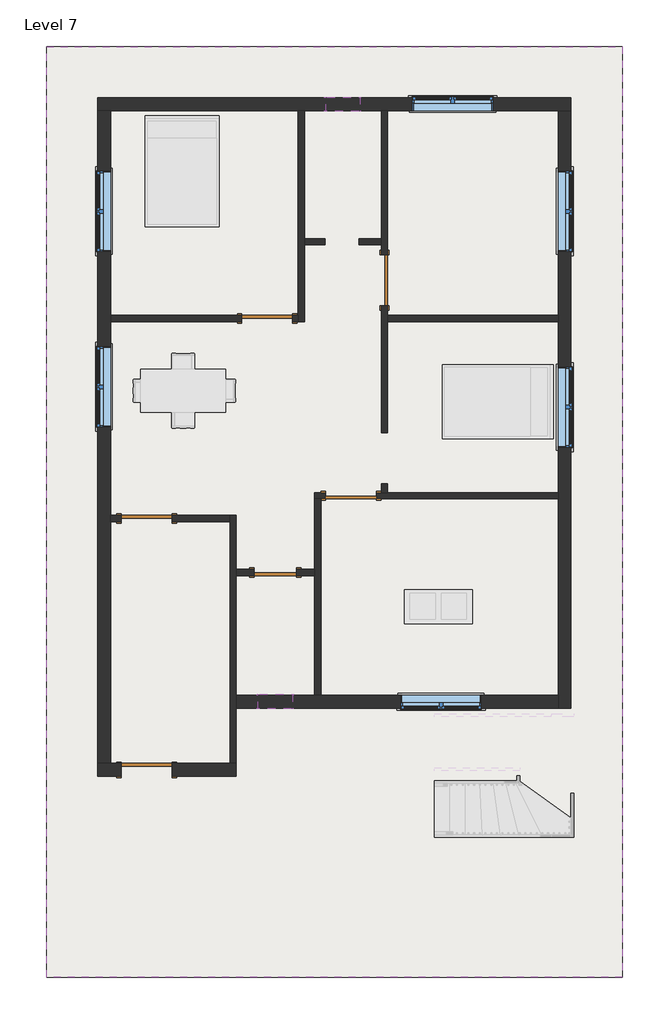
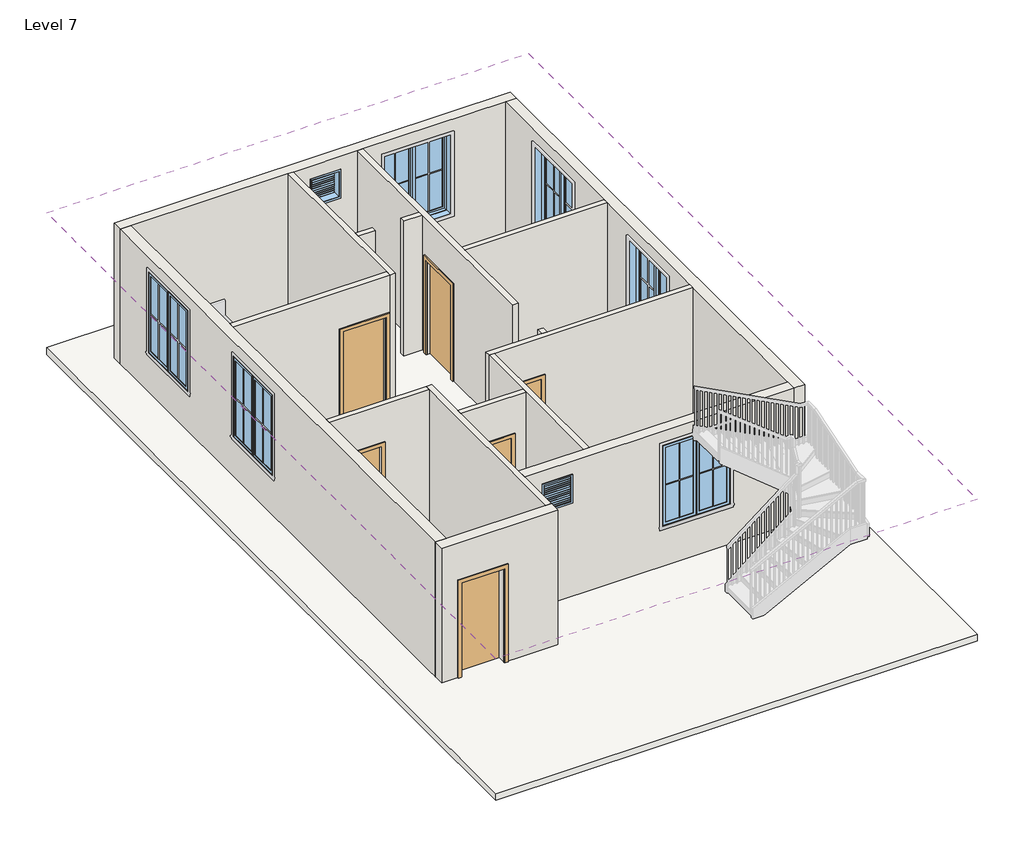
# One storey, part 1 of 3: 17 walls, 8 windows, 6 doors, 2 roofs.
"""IFC4 building model written with IfcOpenShell, lengths in millimetres."""

from ifc_helpers import new_model, si_unit, frame, origin, place, context, project, spatial, polyline, outline, extrude, faceted_brep, transform, mapped, element, save
from components import door_214872d5, single_flush_door_3_e5f9f3c4, single_flush_door_3_305aa2a5, single_flush_door_3_a90ba1ad, window_9ac97e1a, window_f2d8fef0

model = new_model("IFC4")

# Units and contexts
model_context = context("Model", 3, world=origin())
ifc_project = project(units=[si_unit("LENGTHUNIT", "METRE", prefix="MILLI")], contexts=[model_context])

# Site, building, storey
site = spatial("IfcSite", under=ifc_project)
building = spatial("IfcBuilding", under=site)
storey = spatial("IfcBuildingStorey", under=building, Name="Level 7", Elevation=16002.0)

# Doors
placement = place(None, origin())
door_shape = door_214872d5(model_context)
element("IfcDoor", 1, ObjectType="Single-Flush : DOOR 2'6\"", at=placement, inside=storey, context=model_context, shape_type="MappedRepresentation", body=[
    mapped(door_shape, transform((-2309.3144966, -2885.2590409, 16002.0), x_axis=(-1.0, 0.0, 0.0), y_axis=(0.0, -1.0, 0.0), z_axis=(0.0, 0.0, 1.0))),
])
single_flush_door_3_shape = single_flush_door_3_e5f9f3c4(model_context)
element("IfcDoor", 2, ObjectType="Single-Flush : DOOR 3'", at=placement, inside=storey, context=model_context, shape_type="MappedRepresentation", body=[
    mapped(single_flush_door_3_shape, transform((-2455.3644966, 1648.6409591, 16002.0), x_axis=(1.0, 0.0, 0.0), y_axis=(0.0, 1.0, 0.0), z_axis=(0.0, 0.0, 1.0))),
])
element("IfcDoor", 3, ObjectType="Single-Flush : DOOR 3'", at=placement, inside=storey, context=model_context, shape_type="MappedRepresentation", body=[
    mapped(single_flush_door_3_shape, transform((-359.8644966, 2334.4409591, 16002.0), x_axis=(0.0, -1.0, 0.0), y_axis=(1.0, 0.0, 0.0), z_axis=(0.0, 0.0, 1.0))),
])
element("IfcDoor", 4, ObjectType="Single-Flush : DOOR 3'", at=placement, inside=storey, context=model_context, shape_type="MappedRepresentation", body=[
    mapped(single_flush_door_3_shape, transform((-956.7644966, -1513.6590409, 16002.0), x_axis=(-1.0, 0.0, 0.0), y_axis=(0.0, -1.0, 0.0), z_axis=(0.0, 0.0, 1.0))),
])
single_flush_door_3_2_shape = single_flush_door_3_305aa2a5(model_context)
element("IfcDoor", 5, ObjectType="Single-Flush : DOOR 3'", at=placement, inside=storey, context=model_context, shape_type="MappedRepresentation", body=[
    mapped(single_flush_door_3_2_shape, transform((-4608.0144966, -1920.0590409, 16002.0), x_axis=(-1.0, 0.0, 0.0), y_axis=(0.0, -1.0, 0.0), z_axis=(0.0, 0.0, 1.0))),
])
single_flush_door_3_3_shape = single_flush_door_3_a90ba1ad(model_context)
element("IfcDoor", 6, ObjectType="Single-Flush : DOOR 3'", at=placement, inside=storey, context=model_context, shape_type="MappedRepresentation", body=[
    mapped(single_flush_door_3_3_shape, transform((-4608.0144966, -6409.5090409, 16002.0), x_axis=(-1.0, 0.0, 0.0), y_axis=(0.0, -1.0, 0.0), z_axis=(0.0, 0.0, 1.0))),
])

# Roofs
element("IfcRoof", 7, ObjectType="ROOF 6\"", at=placement, inside=storey, context=model_context, shape_type="SweptSolid", body=[
    extrude(outline(polyline([(-6398.7144966, 6506.3909591), (3888.2855034, 6506.3909591), (3888.2855034, -10115.6142473), (-6398.7144966, -10115.6142473), (-6398.7144966, 6506.3909591)])), frame((0.0, 0.0, 15849.6), z_axis=(0.0, 0.0, 1.0), x_axis=(1.0, 0.0, 0.0)), (0.0, 0.0, 1.0), 152.4),
])
element("IfcRoof", 8, ObjectType="ROOF 6\"", at=placement, inside=storey, context=model_context, shape_type="SweptSolid", body=[
    extrude(outline(polyline([(-6398.7144966, 6506.3909591), (3888.2855034, 6506.3909591), (3888.2855034, -10115.6142473), (-6398.7144966, -10115.6142473), (-6398.7144966, 6506.3909591)])), frame((0.0, 0.0, 19050.0), z_axis=(0.0, 0.0, 1.0), x_axis=(1.0, 0.0, 0.0)), (0.0, 0.0, 1.0), 152.4),
])

# Walls
element("IfcWall", 9, ObjectType="WALL 4.5\"", at=placement, inside=storey, context=model_context, shape_type="Brep", body=[
    faceted_brep([(-1902.9144966, 5363.3909591, 16002.0), (-1902.9144966, 1705.7909591, 16002.0), (-1902.9144966, 1591.4909591, 16002.0), (-1902.9144966, 1591.4909591, 19050.0), (-1902.9144966, 1705.7909591, 19050.0), (-1902.9144966, 5363.3909591, 19050.0), (-1788.6144966, 5363.3909591, 16002.0), (-1788.6144966, 5363.3909591, 19050.0), (-1788.6144966, 3077.3909591, 19050.0), (-1788.6144966, 2963.0909591, 19050.0), (-1788.6144966, 1591.4909591, 19050.0), (-1788.6144966, 1591.4909591, 16002.0), (-1788.6144966, 2963.0909591, 16002.0), (-1788.6144966, 3077.3909591, 16002.0)], [[[0, 1, 2, 3, 4, 5]], [[6, 7, 8, 9, 10, 11, 12, 13]], [[2, 1, 0, 6, 13, 12, 11]], [[0, 5, 7, 6]], [[3, 2, 11, 10]], [[5, 4, 3, 10, 9, 8, 7]]]),
])
element("IfcWall", 10, ObjectType="WALL 4.5\"", at=placement, inside=storey, context=model_context, shape_type="SweptSolid", body=[
    extrude(outline(polyline([(18135.6, -1998.1644966), (16002.0, -1998.1644966), (16002.0, -1902.9144966), (19050.0, -1902.9144966), (19050.0, -5255.7144966), (16002.0, -5255.7144966), (16002.0, -2912.5644966), (18135.6, -2912.5644966), (18135.6, -1998.1644966)])), frame((0.0, 1591.4909591, 0.0), z_axis=(0.0, 1.0, 0.0), x_axis=(0.0, 0.0, 1.0)), (0.0, 0.0, 1.0), 114.3),
])
element("IfcWall", 11, ObjectType="WALL 4.5\"", at=placement, inside=storey, context=model_context, shape_type="Brep", body=[
    faceted_brep([(-417.0144966, 1877.2409591, 18135.6), (-417.0144966, 1877.2409591, 16002.0), (-417.0144966, -389.7090409, 16002.0), (-417.0144966, -389.7090409, 19050.0), (-417.0144966, 2963.0909591, 19050.0), (-417.0144966, 3077.3909591, 19050.0), (-417.0144966, 5363.3909591, 19050.0), (-417.0144966, 5363.3909591, 16002.0), (-417.0144966, 3077.3909591, 16002.0), (-417.0144966, 2963.0909591, 16002.0), (-417.0144966, 2791.6409591, 16002.0), (-417.0144966, 2791.6409591, 18135.6), (-302.7144966, -389.7090409, 16002.0), (-302.7144966, 1591.4909591, 16002.0), (-302.7144966, 1705.7909591, 16002.0), (-302.7144966, 1877.2409591, 16002.0), (-302.7144966, 1877.2409591, 18135.6), (-302.7144966, 2791.6409591, 18135.6), (-302.7144966, 2791.6409591, 16002.0), (-302.7144966, 5363.3909591, 16002.0), (-302.7144966, 5363.3909591, 19050.0), (-302.7144966, 1705.7909591, 19050.0), (-302.7144966, 1591.4909591, 19050.0), (-302.7144966, -389.7090409, 19050.0)], [[[0, 1, 2, 3, 4, 5, 6, 7, 8, 9, 10, 11]], [[12, 13, 14, 15, 16, 17, 18, 19, 20, 21, 22, 23]], [[2, 1, 15, 14, 13, 12]], [[10, 9, 8, 7, 19, 18]], [[3, 2, 12, 23]], [[7, 6, 20, 19]], [[16, 15, 1, 0]], [[17, 16, 0, 11]], [[18, 17, 11, 10]], [[6, 5, 4, 3, 23, 22, 21, 20]]]),
])
element("IfcWall", 12, ObjectType="WALL 4.5\"", at=placement, inside=storey, context=model_context, shape_type="SweptSolid", body=[
    extrude(outline(polyline([(-302.7144966, 1705.7909591), (2745.2855034, 1705.7909591), (2745.2855034, 1591.4909591), (-302.7144966, 1591.4909591), (-302.7144966, 1705.7909591)])), frame((0.0, 0.0, 16002.0), z_axis=(0.0, 0.0, 1.0), x_axis=(1.0, 0.0, 0.0)), (0.0, 0.0, 1.0), 3048.0),
])
element("IfcWall", 13, ObjectType="WALL 4.5\"", at=placement, inside=storey, context=model_context, shape_type="SweptSolid", body=[
    extrude(outline(polyline([(-1423.1234474, 2963.0909591), (-1788.6144966, 2963.0909591), (-1788.6144966, 3077.3909591), (-1423.1234474, 3077.3909591), (-1423.1234474, 2963.0909591)])), frame((0.0, 0.0, 16002.0), z_axis=(0.0, 0.0, 1.0), x_axis=(1.0, 0.0, 0.0)), (0.0, 0.0, 1.0), 3048.0),
])
element("IfcWall", 14, ObjectType="WALL 4.5\"", at=placement, inside=storey, context=model_context, shape_type="Brep", body=[
    faceted_brep([(-1413.9644966, -1456.5090409, 18135.6), (-1413.9644966, -1456.5090409, 16002.0), (-1610.8144966, -1456.5090409, 16002.0), (-1610.8144966, -1456.5090409, 19050.0), (-417.0144966, -1456.5090409, 19050.0), (-302.7144966, -1456.5090409, 19050.0), (2745.2855034, -1456.5090409, 19050.0), (2745.2855034, -1456.5090409, 16002.0), (-302.7144966, -1456.5090409, 16002.0), (-417.0144966, -1456.5090409, 16002.0), (-499.5644966, -1456.5090409, 16002.0), (-499.5644966, -1456.5090409, 18135.6), (-1610.8144966, -1570.8090409, 16002.0), (-1496.5144966, -1570.8090409, 16002.0), (-1413.9644966, -1570.8090409, 16002.0), (-1413.9644966, -1570.8090409, 18135.6), (-499.5644966, -1570.8090409, 18135.6), (-499.5644966, -1570.8090409, 16002.0), (2745.2855034, -1570.8090409, 16002.0), (2745.2855034, -1570.8090409, 19050.0), (-1496.5144966, -1570.8090409, 19050.0), (-1610.8144966, -1570.8090409, 19050.0)], [[[0, 1, 2, 3, 4, 5, 6, 7, 8, 9, 10, 11]], [[12, 13, 14, 15, 16, 17, 18, 19, 20, 21]], [[2, 1, 14, 13, 12]], [[10, 9, 8, 7, 18, 17]], [[7, 6, 19, 18]], [[3, 2, 12, 21]], [[15, 14, 1, 0]], [[16, 15, 0, 11]], [[17, 16, 11, 10]], [[6, 5, 4, 3, 21, 20, 19]]]),
])
element("IfcWall", 15, ObjectType="WALL 4.5\"", at=placement, inside=storey, context=model_context, shape_type="SweptSolid", body=[
    extrude(outline(polyline([(-302.7144966, -1304.1090409), (-302.7144966, -1456.5090409), (-417.0144966, -1456.5090409), (-417.0144966, -1304.1090409), (-302.7144966, -1304.1090409)])), frame((0.0, 0.0, 16002.0), z_axis=(0.0, 0.0, 1.0), x_axis=(1.0, 0.0, 0.0)), (0.0, 0.0, 1.0), 3048.0),
])
element("IfcWall", 16, ObjectType="WALL 4.5\"", at=placement, inside=storey, context=model_context, shape_type="Brep", body=[
    faceted_brep([(-1610.8144966, -1570.8090409, 16002.0), (-1610.8144966, -2828.1090409, 16002.0), (-1610.8144966, -2942.4090409, 16002.0), (-1610.8144966, -5076.0090409, 16002.0), (-1610.8144966, -5076.0090409, 19050.0), (-1610.8144966, -2942.4090409, 19050.0), (-1610.8144966, -2828.1090409, 19050.0), (-1610.8144966, -1570.8090409, 19050.0), (-1496.5144966, -1570.8090409, 16002.0), (-1496.5144966, -1570.8090409, 19050.0), (-1496.5144966, -5076.0090409, 19050.0), (-1496.5144966, -5076.0090409, 16002.0)], [[[0, 1, 2, 3, 4, 5, 6, 7]], [[8, 9, 10, 11]], [[3, 2, 1, 0, 8, 11]], [[0, 7, 9, 8]], [[4, 3, 11, 10]], [[7, 6, 5, 4, 10, 9]]]),
])
element("IfcWall", 17, ObjectType="WALL 4.5\"", at=placement, inside=storey, context=model_context, shape_type="SweptSolid", body=[
    extrude(outline(polyline([(16002.0, -3007.8144966), (16002.0, -2690.3144966), (18135.6, -2690.3144966), (18135.6, -1928.3144966), (16002.0, -1928.3144966), (16002.0, -1610.8144966), (19050.0, -1610.8144966), (19050.0, -3007.8144966), (16002.0, -3007.8144966)])), frame((0.0, -2942.4090409, 0.0), z_axis=(0.0, 1.0, 0.0), x_axis=(0.0, 0.0, 1.0)), (0.0, 0.0, 1.0), 114.3),
])
element("IfcWall", 18, ObjectType="WALL 4.5\"", at=placement, inside=storey, context=model_context, shape_type="Brep", body=[
    faceted_brep([(-3007.8144966, -6295.2090409, 16002.0), (-3007.8144966, -5304.6090409, 16002.0), (-3007.8144966, -5076.0090409, 16002.0), (-3007.8144966, -2942.4090409, 16002.0), (-3007.8144966, -2828.1090409, 16002.0), (-3007.8144966, -1862.9090409, 16002.0), (-3007.8144966, -1862.9090409, 19050.0), (-3007.8144966, -2828.1090409, 19050.0), (-3007.8144966, -2942.4090409, 19050.0), (-3007.8144966, -5076.0090409, 19050.0), (-3007.8144966, -5304.6090409, 19050.0), (-3007.8144966, -6295.2090409, 19050.0), (-3122.1144966, -6295.2090409, 16002.0), (-3122.1144966, -6295.2090409, 19050.0), (-3122.1144966, -1977.2090409, 19050.0), (-3122.1144966, -1862.9090409, 19050.0), (-3122.1144966, -1862.9090409, 16002.0), (-3122.1144966, -1977.2090409, 16002.0)], [[[0, 1, 2, 3, 4, 5, 6, 7, 8, 9, 10, 11]], [[12, 13, 14, 15, 16, 17]], [[5, 4, 3, 2, 1, 0, 12, 17, 16]], [[0, 11, 13, 12]], [[6, 5, 16, 15]], [[11, 10, 9, 8, 7, 6, 15, 14, 13]]]),
])
element("IfcWall", 19, ObjectType="WALL 4.5\"", at=placement, inside=storey, context=model_context, shape_type="SweptSolid", body=[
    extrude(outline(polyline([(16002.0, -5255.7144966), (16002.0, -5065.2144966), (18135.6, -5065.2144966), (18135.6, -4150.8144966), (16002.0, -4150.8144966), (16002.0, -3122.1144966), (19050.0, -3122.1144966), (19050.0, -5255.7144966), (16002.0, -5255.7144966)])), frame((0.0, -1977.2090409, 0.0), z_axis=(0.0, 1.0, 0.0), x_axis=(0.0, 0.0, 1.0)), (0.0, 0.0, 1.0), 114.3),
])
element("IfcWall", 20, ObjectType="WALL 4.5\"", at=placement, inside=storey, context=model_context, shape_type="SweptSolid", body=[
    extrude(outline(polyline([(-417.0144966, 2963.0909591), (-814.3659123, 2963.0909591), (-814.3659123, 3077.3909591), (-417.0144966, 3077.3909591), (-417.0144966, 2963.0909591)])), frame((0.0, 0.0, 16002.0), z_axis=(0.0, 0.0, 1.0), x_axis=(1.0, 0.0, 0.0)), (0.0, 0.0, 1.0), 3048.0),
])
element("IfcWall", 21, ObjectType="WALL 9\"", at=placement, inside=storey, context=model_context, shape_type="Brep", body=[
    faceted_brep([(-5484.3144966, 5363.3909591, 16002.0), (-5255.7144966, 5363.3909591, 16002.0), (-1902.9144966, 5363.3909591, 16002.0), (-1788.6144966, 5363.3909591, 16002.0), (-417.0144966, 5363.3909591, 16002.0), (-302.7144966, 5363.3909591, 16002.0), (2745.2855034, 5363.3909591, 16002.0), (2973.8855034, 5363.3909591, 16002.0), (2973.8855034, 5363.3909591, 19050.0), (2745.2855034, 5363.3909591, 19050.0), (-302.7144966, 5363.3909591, 19050.0), (-417.0144966, 5363.3909591, 19050.0), (-1788.6144966, 5363.3909591, 19050.0), (-1902.9144966, 5363.3909591, 19050.0), (-5255.7144966, 5363.3909591, 19050.0), (-5484.3144966, 5363.3909591, 19050.0), (1583.2355034, 5363.3909591, 18745.2), (1583.2355034, 5363.3909591, 16916.4), (135.4355034, 5363.3909591, 16916.4), (135.4355034, 5363.3909591, 18745.2), (-1407.6144966, 5363.3909591, 18745.2), (-798.0144966, 5363.3909591, 18745.2), (-798.0144966, 5363.3909591, 18135.6), (-1407.6144966, 5363.3909591, 18135.6), (-5484.3144966, 5591.9909591, 16002.0), (-5484.3144966, 5591.9909591, 19050.0), (2973.8855034, 5591.9909591, 19050.0), (2973.8855034, 5591.9909591, 16002.0), (1583.2355034, 5591.9909591, 18745.2), (135.4355034, 5591.9909591, 18745.2), (135.4355034, 5591.9909591, 16916.4), (1583.2355034, 5591.9909591, 16916.4), (-1407.6144966, 5591.9909591, 18745.2), (-1407.6144966, 5591.9909591, 18135.6), (-798.0144966, 5591.9909591, 18135.6), (-798.0144966, 5591.9909591, 18745.2)], [[[0, 1, 2, 3, 4, 5, 6, 7, 8, 9, 10, 11, 12, 13, 14, 15], [16, 17, 18, 19], [20, 21, 22, 23]], [[24, 25, 26, 27], [28, 29, 30, 31], [32, 33, 34, 35]], [[7, 6, 5, 4, 3, 2, 1, 0, 24, 27]], [[8, 7, 27, 26]], [[0, 15, 25, 24]], [[17, 16, 28, 31]], [[18, 17, 31, 30]], [[19, 18, 30, 29]], [[16, 19, 29, 28]], [[33, 32, 20, 23]], [[34, 33, 23, 22]], [[35, 34, 22, 21]], [[32, 35, 21, 20]], [[15, 14, 13, 12, 11, 10, 9, 8, 26, 25]]]),
])
element("IfcWall", 22, ObjectType="WALL 9\"", at=placement, inside=storey, context=model_context, shape_type="Brep", body=[
    faceted_brep([(2745.2855034, 5363.3909591, 16002.0), (2745.2855034, 1705.7909591, 16002.0), (2745.2855034, 1591.4909591, 16002.0), (2745.2855034, -1456.5090409, 16002.0), (2745.2855034, -1570.8090409, 16002.0), (2745.2855034, -5076.0090409, 16002.0), (2745.2855034, -5304.6090409, 16002.0), (2745.2855034, -5304.6090409, 19050.0), (2745.2855034, -5076.0090409, 19050.0), (2745.2855034, -1570.8090409, 19050.0), (2745.2855034, -1456.5090409, 19050.0), (2745.2855034, 1591.4909591, 19050.0), (2745.2855034, 1705.7909591, 19050.0), (2745.2855034, 5363.3909591, 19050.0), (2745.2855034, -656.4090409, 18745.2), (2745.2855034, -656.4090409, 16916.4), (2745.2855034, 791.3909591, 16916.4), (2745.2855034, 791.3909591, 18745.2), (2745.2855034, 2839.2659591, 18745.2), (2745.2855034, 2839.2659591, 16916.4), (2745.2855034, 4287.0659591, 16916.4), (2745.2855034, 4287.0659591, 18745.2), (2973.8855034, 5363.3909591, 16002.0), (2973.8855034, 5363.3909591, 19050.0), (2973.8855034, -5304.6090409, 19050.0), (2973.8855034, -5304.6090409, 16002.0), (2973.8855034, -656.4090409, 18745.2), (2973.8855034, 791.3909591, 18745.2), (2973.8855034, 791.3909591, 16916.4), (2973.8855034, -656.4090409, 16916.4), (2973.8855034, 2839.2659591, 18745.2), (2973.8855034, 4287.0659591, 18745.2), (2973.8855034, 4287.0659591, 16916.4), (2973.8855034, 2839.2659591, 16916.4)], [[[0, 1, 2, 3, 4, 5, 6, 7, 8, 9, 10, 11, 12, 13], [14, 15, 16, 17], [18, 19, 20, 21]], [[22, 23, 24, 25], [26, 27, 28, 29], [30, 31, 32, 33]], [[6, 5, 4, 3, 2, 1, 0, 22, 25]], [[0, 13, 23, 22]], [[7, 6, 25, 24]], [[15, 14, 26, 29]], [[16, 15, 29, 28]], [[17, 16, 28, 27]], [[14, 17, 27, 26]], [[19, 18, 30, 33]], [[20, 19, 33, 32]], [[21, 20, 32, 31]], [[18, 21, 31, 30]], [[13, 12, 11, 10, 9, 8, 7, 24, 23]]]),
])
element("IfcWall", 23, ObjectType="WALL 9\"", at=placement, inside=storey, context=model_context, shape_type="Brep", body=[
    faceted_brep([(2745.2855034, -5076.0090409, 16002.0), (-1496.5144966, -5076.0090409, 16002.0), (-1610.8144966, -5076.0090409, 16002.0), (-3007.8144966, -5076.0090409, 16002.0), (-3007.8144966, -5076.0090409, 19050.0), (-1610.8144966, -5076.0090409, 19050.0), (-1496.5144966, -5076.0090409, 19050.0), (2745.2855034, -5076.0090409, 19050.0), (-70.9394966, -5076.0090409, 18745.2), (-70.9394966, -5076.0090409, 16916.4), (1376.8605034, -5076.0090409, 16916.4), (1376.8605034, -5076.0090409, 18745.2), (-2004.5144966, -5076.0090409, 18745.2), (-2614.1144966, -5076.0090409, 18745.2), (-2614.1144966, -5076.0090409, 18135.6), (-2004.5144966, -5076.0090409, 18135.6), (2745.2855034, -5304.6090409, 16002.0), (2745.2855034, -5304.6090409, 19050.0), (-3007.8144966, -5304.6090409, 19050.0), (-3007.8144966, -5304.6090409, 16002.0), (-70.9394966, -5304.6090409, 18745.2), (1376.8605034, -5304.6090409, 18745.2), (1376.8605034, -5304.6090409, 16916.4), (-70.9394966, -5304.6090409, 16916.4), (-2004.5144966, -5304.6090409, 18745.2), (-2004.5144966, -5304.6090409, 18135.6), (-2614.1144966, -5304.6090409, 18135.6), (-2614.1144966, -5304.6090409, 18745.2)], [[[0, 1, 2, 3, 4, 5, 6, 7], [8, 9, 10, 11], [12, 13, 14, 15]], [[16, 17, 18, 19], [20, 21, 22, 23], [24, 25, 26, 27]], [[3, 2, 1, 0, 16, 19]], [[0, 7, 17, 16]], [[4, 3, 19, 18]], [[9, 8, 20, 23]], [[10, 9, 23, 22]], [[11, 10, 22, 21]], [[8, 11, 21, 20]], [[25, 24, 12, 15]], [[26, 25, 15, 14]], [[27, 26, 14, 13]], [[24, 27, 13, 12]], [[7, 6, 5, 4, 18, 17]]]),
])
element("IfcWall", 24, ObjectType="WALL 9\"", at=placement, inside=storey, context=model_context, shape_type="Brep", body=[
    faceted_brep([(-5065.2144966, -6295.2090409, 18135.6), (-5065.2144966, -6295.2090409, 16002.0), (-5255.7144966, -6295.2090409, 16002.0), (-5484.3144966, -6295.2090409, 16002.0), (-5484.3144966, -6295.2090409, 19050.0), (-5255.7144966, -6295.2090409, 19050.0), (-3122.1144966, -6295.2090409, 19050.0), (-3007.8144966, -6295.2090409, 19050.0), (-3007.8144966, -6295.2090409, 16002.0), (-3122.1144966, -6295.2090409, 16002.0), (-4150.8144966, -6295.2090409, 16002.0), (-4150.8144966, -6295.2090409, 18135.6), (-5484.3144966, -6523.8090409, 16002.0), (-5065.2144966, -6523.8090409, 16002.0), (-5065.2144966, -6523.8090409, 18135.6), (-4150.8144966, -6523.8090409, 18135.6), (-4150.8144966, -6523.8090409, 16002.0), (-3007.8144966, -6523.8090409, 16002.0), (-3007.8144966, -6523.8090409, 19050.0), (-5484.3144966, -6523.8090409, 19050.0)], [[[0, 1, 2, 3, 4, 5, 6, 7, 8, 9, 10, 11]], [[12, 13, 14, 15, 16, 17, 18, 19]], [[10, 9, 8, 17, 16]], [[3, 2, 1, 13, 12]], [[4, 3, 12, 19]], [[8, 7, 18, 17]], [[7, 6, 5, 4, 19, 18]], [[14, 13, 1, 0]], [[15, 14, 0, 11]], [[16, 15, 11, 10]]]),
])
element("IfcWall", 25, ObjectType="WALL 9\"", at=placement, inside=storey, context=model_context, shape_type="Brep", body=[
    faceted_brep([(-5255.7144966, -6295.2090409, 16002.0), (-5255.7144966, -1977.2090409, 16002.0), (-5255.7144966, -1862.9090409, 16002.0), (-5255.7144966, 1591.4909591, 16002.0), (-5255.7144966, 1705.7909591, 16002.0), (-5255.7144966, 5363.3909591, 16002.0), (-5255.7144966, 5363.3909591, 19050.0), (-5255.7144966, 1705.7909591, 19050.0), (-5255.7144966, 1591.4909591, 19050.0), (-5255.7144966, -1862.9090409, 19050.0), (-5255.7144966, -1977.2090409, 19050.0), (-5255.7144966, -6295.2090409, 19050.0), (-5255.7144966, 4287.0659591, 18745.2), (-5255.7144966, 4287.0659591, 16916.4), (-5255.7144966, 2839.2659591, 16916.4), (-5255.7144966, 2839.2659591, 18745.2), (-5255.7144966, 1153.3409591, 18745.2), (-5255.7144966, 1153.3409591, 16916.4), (-5255.7144966, -294.4590409, 16916.4), (-5255.7144966, -294.4590409, 18745.2), (-5484.3144966, -6295.2090409, 16002.0), (-5484.3144966, -6295.2090409, 19050.0), (-5484.3144966, 5363.3909591, 19050.0), (-5484.3144966, 5363.3909591, 16002.0), (-5484.3144966, 4287.0659591, 18745.2), (-5484.3144966, 2839.2659591, 18745.2), (-5484.3144966, 2839.2659591, 16916.4), (-5484.3144966, 4287.0659591, 16916.4), (-5484.3144966, 1153.3409591, 18745.2), (-5484.3144966, -294.4590409, 18745.2), (-5484.3144966, -294.4590409, 16916.4), (-5484.3144966, 1153.3409591, 16916.4)], [[[0, 1, 2, 3, 4, 5, 6, 7, 8, 9, 10, 11], [12, 13, 14, 15], [16, 17, 18, 19]], [[20, 21, 22, 23], [24, 25, 26, 27], [28, 29, 30, 31]], [[5, 4, 3, 2, 1, 0, 20, 23]], [[0, 11, 21, 20]], [[6, 5, 23, 22]], [[13, 12, 24, 27]], [[14, 13, 27, 26]], [[15, 14, 26, 25]], [[12, 15, 25, 24]], [[17, 16, 28, 31]], [[18, 17, 31, 30]], [[19, 18, 30, 29]], [[16, 19, 29, 28]], [[11, 10, 9, 8, 7, 6, 22, 21]]]),
])

# Windows
window_shape = window_9ac97e1a(model_context)
element("IfcWindow", 26, ObjectType="Window-Casement-Double : 57\" x 72\"", at=placement, inside=storey, context=model_context, shape_type="MappedRepresentation", body=[
    mapped(window_shape, transform((2859.5855034, 67.4909591, 16002.0), x_axis=(0.0, -1.0, 0.0), y_axis=(1.0, 0.0, 0.0), z_axis=(0.0, 0.0, 1.0))),
])
element("IfcWindow", 27, ObjectType="Window-Casement-Double : 57\" x 72\"", at=placement, inside=storey, context=model_context, shape_type="MappedRepresentation", body=[
    mapped(window_shape, transform((2859.5855034, 3563.1659591, 16002.0), x_axis=(0.0, -1.0, 0.0), y_axis=(1.0, 0.0, 0.0), z_axis=(0.0, 0.0, 1.0))),
])
element("IfcWindow", 28, ObjectType="Window-Casement-Double : 57\" x 72\"", at=placement, inside=storey, context=model_context, shape_type="MappedRepresentation", body=[
    mapped(window_shape, transform((859.3355034, 5477.6909591, 16002.0), x_axis=(1.0, 0.0, 0.0), y_axis=(0.0, 1.0, 0.0), z_axis=(0.0, 0.0, 1.0))),
])
element("IfcWindow", 29, ObjectType="Window-Casement-Double : 57\" x 72\"", at=placement, inside=storey, context=model_context, shape_type="MappedRepresentation", body=[
    mapped(window_shape, transform((-5370.0144966, 3563.1659591, 16002.0), x_axis=(0.0, 1.0, 0.0), y_axis=(-1.0, 0.0, 0.0), z_axis=(0.0, 0.0, 1.0))),
])
element("IfcWindow", 30, ObjectType="Window-Casement-Double : 57\" x 72\"", at=placement, inside=storey, context=model_context, shape_type="MappedRepresentation", body=[
    mapped(window_shape, transform((-5370.0144966, 429.4409591, 16002.0), x_axis=(0.0, 1.0, 0.0), y_axis=(-1.0, 0.0, 0.0), z_axis=(0.0, 0.0, 1.0))),
])
element("IfcWindow", 31, ObjectType="Window-Casement-Double : 57\" x 72\"", at=placement, inside=storey, context=model_context, shape_type="MappedRepresentation", body=[
    mapped(window_shape, transform((652.9605034, -5190.3090409, 16002.0), x_axis=(-1.0, 0.0, 0.0), y_axis=(0.0, -1.0, 0.0), z_axis=(0.0, 0.0, 1.0))),
])
window_2_shape = window_f2d8fef0(model_context)
element("IfcWindow", 32, ObjectType="Window-Louvers : 24\" x 24\"", at=placement, inside=storey, context=model_context, shape_type="MappedRepresentation", body=[
    mapped(window_2_shape, transform((-1102.8144966, 5484.0409591, 17221.2), x_axis=(1.0, 0.0, 0.0), y_axis=(0.0, 1.0, 0.0), z_axis=(0.0, 0.0, 1.0))),
])
element("IfcWindow", 33, ObjectType="Window-Louvers : 24\" x 24\"", at=placement, inside=storey, context=model_context, shape_type="MappedRepresentation", body=[
    mapped(window_2_shape, transform((-2309.3144966, -5196.6590409, 17221.2), x_axis=(-1.0, 0.0, 0.0), y_axis=(0.0, -1.0, 0.0), z_axis=(0.0, 0.0, 1.0))),
])

save(model, "model.ifc")

# Revit data of these elements
# Type "Single-Flush : DOOR 2'6\""
#   Type Mark = "10"
#   Construction Type Id = "MDOOR"
#   Assembly Code = "C1020"
#   Analytic Construction = "Metal"
#   Thickness = 0' - 2"
#   Heat Transfer Coefficient (U) = 0.651978 BTU/(h·ft²·°F)
#   Height = 7' - 0"
#   Trim Projection Ext = 0' - 1"
#   Trim Projection Int = 0' - 1"
#   Trim Width = 0' - 3"
#   Width = 2' - 6"
#   Define Thermal Properties by = 1
#   Door Material = Door - Panel
#   Frame Material = Door - Frame
#   Visual Light Transmittance = 0
#   Solar Heat Gain Coefficient = 0
#   Function = (empty or 0)
#   Wall Closure = (empty or 0)
# Type "Single-Flush : DOOR 3'"
#   Type Mark = "9"
#   Construction Type Id = "MDOOR"
#   Assembly Code = "C1020"
#   Analytic Construction = "Metal"
#   Thickness = 0' - 2"
#   Heat Transfer Coefficient (U) = 0.651978 BTU/(h·ft²·°F)
#   Height = 7' - 0"
#   Trim Projection Ext = 0' - 1"
#   Trim Projection Int = 0' - 1"
#   Trim Width = 0' - 3"
#   Width = 3' - 0"
#   Define Thermal Properties by = 1
#   Door Material = Door - Panel
#   Frame Material = Door - Frame
#   Visual Light Transmittance = 0
#   Solar Heat Gain Coefficient = 0
#   Function = (empty or 0)
#   Wall Closure = (empty or 0)
# Type "ROOF 6\""
#   Assembly Code = "B1020"
#   Layers, outside or top first: 0' - 6" no material (function 1)
# Type "WALL 4.5\""
#   Assembly Code = "B2010"
#   Layers, outside or top first: 0' - 4 1/2" no material (function 1)
# Type "WALL 9\""
#   Assembly Code = "B2010"
#   Layers, outside or top first: 0' - 9" no material (function 1)
# Type "Window-Casement-Double : 57\" x 72\""
#   Type Mark = "17"
#   Fire Rating = "0.5h"
#   Assembly Code = "B2020100"
#   Analytic Construction = "Double glazing - domestic"
#   Frame Extension [instance default] = 0' - 0 1/4"
#   Window Inset [instance default] = 0' - 0"
#   Wall Thickness [instance default] = 0' - 6"
#   Interior Wall Closure [instance default] = 0' - 2 1/4"
#   Half Width = 2' - 4 1/2"
#   Visual Light Transmittance = 0.81
#   Thermal Resistance (R) = 1.8146 (h·ft²·°F)/BTU
#   Solar Heat Gain Coefficient = 0.76
#   Rough Width = 4' - 9 1/2"
#   Rough Height = 6' - 0 1/2"
#   Height = 6' - 0"
#   Heat Transfer Coefficient (U) = 0.5511 BTU/(h·ft²·°F)
#   Exterior Wall Closure [instance default] = 0' - 1 1/4"
#   Extension Jamb [instance default] = 0' - 2 1/4"
#   Default Sill Height = 3' - 0"
#   Width = 4' - 9"
#   Define Thermal Properties by = 0
#   Muntin Visibility = yes
#   Interior Trim Visibility [instance default] = yes
#   Exterior Trim Visibility [instance default] = yes
#   Extension Jamb Visibility [instance default] = yes
#   Interior Trim Material = Wood - Stained
#   Muntin Pattern = Muntin Pattern_2x2 : Muntin Pattern_2x2
#   Interior Trim = Trim-Window-Interior-Flat : Picture Frame
#   Interior Frame Material = Wood - Stained
#   Glass Panel Material = Glass
#   Exterior Trim Material = Clad - White
#   Exterior Trim = Trim-Window-Exterior-Flat : with Sill
#   Exterior Frame Material = Clad - White
#   Wall Closure = (empty or 0)
# Type "Window-Louvers : 24\" x 24\""
#   Type Mark = "18"
#   Construction Type Id = "GSP4R"
#   Assembly Code = "B20"
#   Analytic Construction = "1/8 in Pilkington single glazing"
#   Visual Light Transmittance = 0.9
#   Thermal Resistance (R) = 1.53941 (h·ft²·°F)/BTU
#   Solar Heat Gain Coefficient = 0.78
#   Max Height = 1' - 11.74264"
#   Height = 2' - 0"
#   Heat Transfer Coefficient (U) = 0.6496 BTU/(h·ft²·°F)
#   Blade Width [instance default] = 1' - 10 1/2"
#   Blade Vertical Thickness = 0' - 0.35355"
#   Blade Thickness = 0' - 0 1/4"
#   Blade Spacing = 0' - 1 1/2"
#   Blade Height = 0' - 1.85355"
#   Blade Depth = 0' - 3"
#   Blade Angle = 45.00°
#   Default Sill Height = 3' - 0"
#   Trim Projection_Exterior = 0' - 0 1/2"
#   Trim Projection_Interior = 0' - 0 1/2"
#   Trim Width_Exterior = 0' - 1 1/2"
#   Trim Width_Interior = 0' - 1 1/2"
#   Width = 2' - 0"
#   Max Blade Count = 12
#   Define Thermal Properties by = 1
#   Blade Count = 12
#   Frame Material = Birch
#   Louver Material = Birch
#   Trim Exterior Material = Birch
#   Trim Interior Material = Birch
#   Wall Closure = (empty or 0)
# Element 1 (IfcDoor, "Single-Flush : DOOR 2'6\"")
#   Phase Created = New Construction
#   Materials on its faces: "Door - Frame", "Door - Panel"
# Elements 2, 3, 4, 5, 6 (IfcDoor, "Single-Flush : DOOR 3'")
#   Phase Created = New Construction
#   Materials on its faces: "Door - Frame", "Door - Panel"
# Element 7 (IfcRoof, "ROOF 6\"")
#   built-in parameter 1001705 = 52.5 (stored number, unit not read)
#   built-in parameter 1001701 = -0.5 (stored number, unit not read)
#   built-in parameter 1001710 = 33615
#   Phase Created = New Construction
#   Materials on its faces: "Cherry", "Default Roof", "Softwood, Lumber"
# Element 8 (IfcRoof, "ROOF 6\"")
#   built-in parameter 1001705 = 63 (stored number, unit not read)
#   built-in parameter 1001701 = 10 (stored number, unit not read)
#   built-in parameter 1001710 = 33615
#   Phase Created = New Construction
#   Materials on its faces: "Cherry", "Default Roof", "Softwood, Lumber"
# Elements 9, 10, 11, 12, 13, 14, 15, 16, 17, 18, 19, 20 (IfcWall, "WALL 4.5\"")
#   Top Offset = 0' - 0"
#   Base Offset = 0' - 0"
#   Unconnected Height = 10' - 0"
#   wall height = 10' - 0"
#   Phase Created = New Construction
#   Base Constraint = Level 7
#   Materials on its faces: "Default Wall"
# Elements 21, 22, 23, 24, 25 (IfcWall, "WALL 9\"")
#   Top Offset = 0' - 0"
#   Base Offset = 0' - 0"
#   Unconnected Height = 10' - 0"
#   wall height = 10' - 0"
#   Phase Created = New Construction
#   Base Constraint = Level 7
#   Materials on its faces: "Default Wall"
# Element 26 (IfcWindow, "Window-Casement-Double : 57\" x 72\"")
#   Mark = "41"
#   Window Inset = 0' - 0"
#   Interior Wall Closure = 0' - 2 1/4"
#   Frame Extension = 0' - 0 1/4"
#   Exterior Wall Closure = 0' - 1 1/4"
#   Interior Trim Visibility = yes
#   Exterior Trim Visibility = yes
#   Phase Created = New Construction
#   Materials on its faces: "Wood - Stained", "Glass", "Clad - White"
# Element 27 (IfcWindow, "Window-Casement-Double : 57\" x 72\"")
#   Mark = "42"
#   Window Inset = 0' - 0"
#   Interior Wall Closure = 0' - 2 1/4"
#   Frame Extension = 0' - 0 1/4"
#   Exterior Wall Closure = 0' - 1 1/4"
#   Interior Trim Visibility = yes
#   Exterior Trim Visibility = yes
#   Phase Created = New Construction
#   Materials on its faces: "Wood - Stained", "Glass", "Clad - White"
# Element 28 (IfcWindow, "Window-Casement-Double : 57\" x 72\"")
#   Mark = "43"
#   Window Inset = 0' - 0"
#   Interior Wall Closure = 0' - 2 1/4"
#   Frame Extension = 0' - 0 1/4"
#   Exterior Wall Closure = 0' - 1 1/4"
#   Interior Trim Visibility = yes
#   Exterior Trim Visibility = yes
#   Phase Created = New Construction
#   Materials on its faces: "Wood - Stained", "Glass", "Clad - White"
# Element 29 (IfcWindow, "Window-Casement-Double : 57\" x 72\"")
#   Mark = "44"
#   Window Inset = 0' - 0"
#   Interior Wall Closure = 0' - 2 1/4"
#   Frame Extension = 0' - 0 1/4"
#   Exterior Wall Closure = 0' - 1 1/4"
#   Interior Trim Visibility = yes
#   Exterior Trim Visibility = yes
#   Phase Created = New Construction
#   Materials on its faces: "Wood - Stained", "Glass", "Clad - White"
# Element 30 (IfcWindow, "Window-Casement-Double : 57\" x 72\"")
#   Mark = "45"
#   Window Inset = 0' - 0"
#   Interior Wall Closure = 0' - 2 1/4"
#   Frame Extension = 0' - 0 1/4"
#   Exterior Wall Closure = 0' - 1 1/4"
#   Interior Trim Visibility = yes
#   Exterior Trim Visibility = yes
#   Phase Created = New Construction
#   Materials on its faces: "Wood - Stained", "Glass", "Clad - White"
# Element 31 (IfcWindow, "Window-Casement-Double : 57\" x 72\"")
#   Mark = "46"
#   Window Inset = 0' - 0"
#   Interior Wall Closure = 0' - 2 1/4"
#   Frame Extension = 0' - 0 1/4"
#   Exterior Wall Closure = 0' - 1 1/4"
#   Interior Trim Visibility = yes
#   Exterior Trim Visibility = yes
#   Phase Created = New Construction
#   Materials on its faces: "Wood - Stained", "Glass", "Clad - White"
# Element 32 (IfcWindow, "Window-Louvers : 24\" x 24\"")
#   Mark = "47"
#   Blade Width = 1' - 10 1/2"
#   Phase Created = New Construction
#   Materials on its faces: "Birch"
# Element 33 (IfcWindow, "Window-Louvers : 24\" x 24\"")
#   Mark = "48"
#   Blade Width = 1' - 10 1/2"
#   Phase Created = New Construction
#   Materials on its faces: "Birch"
# Materials
#   "Door - Panel": class "Wood", colour RGB 210 159 95, transparency 0, Cost = 0
#   "Door - Frame": colour RGB 118 70 51, transparency 0, Cost = 0
#   "Wood - Stained": class "Wood", colour RGB 224 178 126, transparency 0, Cost = 0
#   "Glass": class "Glass", colour RGB 0 128 192, transparency 0.75, Description = "Soda Lime Glass", Cost = 0
#   "Clad - White": class "Wood", colour RGB 242 242 238, transparency 0, Cost = 0
#   "Birch": class "Wood", colour RGB 224 178 126, transparency 0, Description = "Betula Alleghaniensis", Cost = 0
#   "Cherry": class "Wood", colour RGB 226 177 128, transparency 0, Description = "Prunus Serotina", Cost = 0
#   "Default Roof": colour RGB 88 101 114, transparency 0, Cost = 0
#   "Softwood, Lumber": class "Wood", colour RGB 223 192 134, transparency 0, Description = "Pinus Echinata", Cost = 0
#   "Default Wall": colour RGB 128 128 128, transparency 0, Cost = 0
